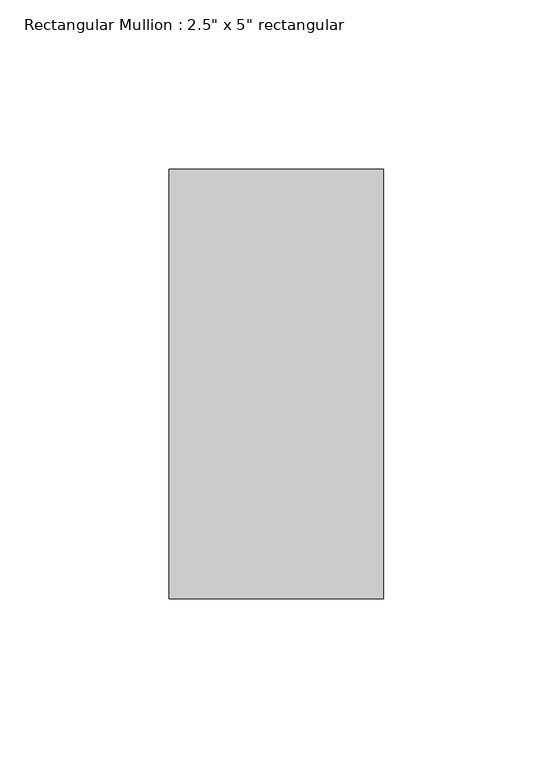
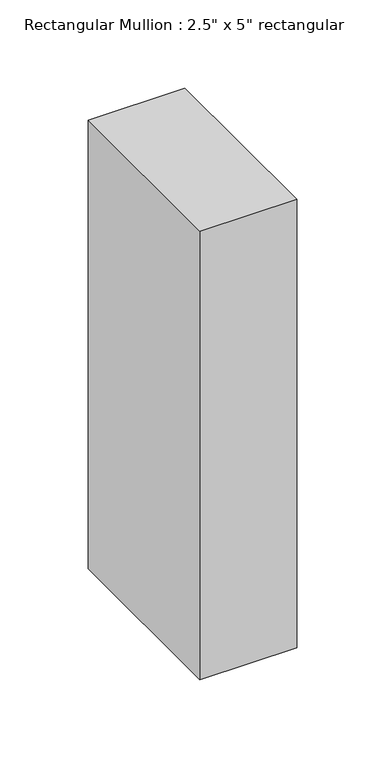
"""IFC4 building model written with IfcOpenShell, lengths in millimetres: member geometry."""

from ifc_helpers import new_model, si_unit, frame, origin, place, context, project, spatial, polyline, outline, extrude, source, transform, mapped, element, save


def member_9850ab14(model_context):
    return source(origin(), model_context, "Body", "SweptSolid", [
        extrude(outline(polyline([(31.75, 63.5), (31.75, -63.5), (-31.75, -63.5), (-31.75, 63.5), (31.75, 63.5)])), frame((0.0, 0.0, -311.15), z_axis=(0.0, 0.0, 1.0), x_axis=(1.0, 0.0, 0.0)), (0.0, 0.0, 1.0), 311.15),
    ])


if __name__ == "__main__":
    model = new_model("IFC4")
    model_context = context("Model", 3, world=origin())
    ifc_project = project(units=[si_unit("LENGTHUNIT", "METRE", prefix="MILLI")], contexts=[model_context])
    site = spatial("IfcSite", under=ifc_project)
    building = spatial("IfcBuilding", under=site)
    placement = place(None, origin())
    member_shape = member_9850ab14(model_context)
    element("IfcMember", 1, ObjectType="Rectangular Mullion : 2.5\" x 5\" rectangular", at=placement, inside=building, context=model_context, shape_type="MappedRepresentation", body=[
        mapped(member_shape, transform((0.0, 0.0, 0.0), x_axis=(1.0, 0.0, 0.0), y_axis=(0.0, 1.0, 0.0), z_axis=(0.0, 0.0, 1.0))),
    ])
    save(model, "model.ifc")

# Revit data of these elements
# Type "Rectangular Mullion : 2.5\" x 5\" rectangular"
#   built-in parameter 1007304 = 0.416667 (stored number, unit not read)
#   built-in parameter 1007301 = 0.104167 (stored number, unit not read)
#   built-in parameter 1007300 = 0.104167 (stored number, unit not read)
